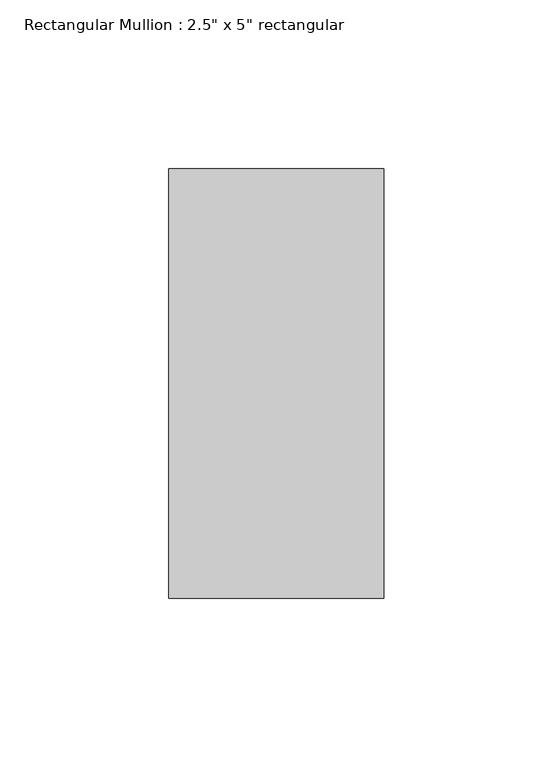
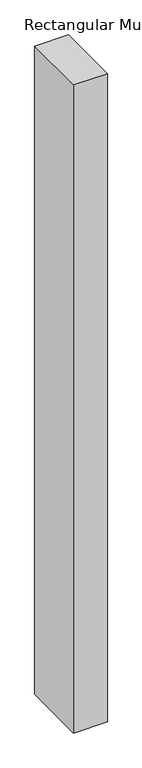
"""IFC4 building model written with IfcOpenShell, lengths in millimetres: member geometry."""

from ifc_helpers import new_model, si_unit, frame, origin, place, context, project, spatial, polyline, outline, extrude, source, transform, mapped, element, save


def member_acf158a7(model_context):
    return source(origin(), model_context, "Body", "SweptSolid", [
        extrude(outline(polyline([(0.0, 63.5), (0.0, -63.5), (-63.5, -63.5), (-63.5, 63.5), (0.0, 63.5)])), frame((0.0, 0.0, -1290.6993822), z_axis=(0.0, 0.0, 1.0), x_axis=(1.0, 0.0, 0.0)), (0.0, 0.0, 1.0), 1290.6993822),
    ])


if __name__ == "__main__":
    model = new_model("IFC4")
    model_context = context("Model", 3, world=origin())
    ifc_project = project(units=[si_unit("LENGTHUNIT", "METRE", prefix="MILLI")], contexts=[model_context])
    site = spatial("IfcSite", under=ifc_project)
    building = spatial("IfcBuilding", under=site)
    placement = place(None, origin())
    member_shape = member_acf158a7(model_context)
    element("IfcMember", 1, ObjectType="Rectangular Mullion : 2.5\" x 5\" rectangular", at=placement, inside=building, context=model_context, shape_type="MappedRepresentation", body=[
        mapped(member_shape, transform((0.0, 0.0, 0.0), x_axis=(1.0, 0.0, 0.0), y_axis=(0.0, 1.0, 0.0), z_axis=(0.0, 0.0, 1.0))),
    ])
    save(model, "model.ifc")

# Revit data of these elements
# Type "Rectangular Mullion : 2.5\" x 5\" rectangular"
#   built-in parameter 1007304 = 0.416667 (stored number, unit not read)
#   built-in parameter 1007301 = 0.104167 (stored number, unit not read)
#   built-in parameter 1007300 = 0.104167 (stored number, unit not read)
# Element 1 (IfcMember, "Rectangular Mullion : 2.5\" x 5\" rectangular")
#   Materials on its faces: "Aluminum"
# Materials
#   "Aluminum": class "Metal", colour RGB 247 247 247, transparency 0, Description = "Aluminum 6061", Cost = 0
